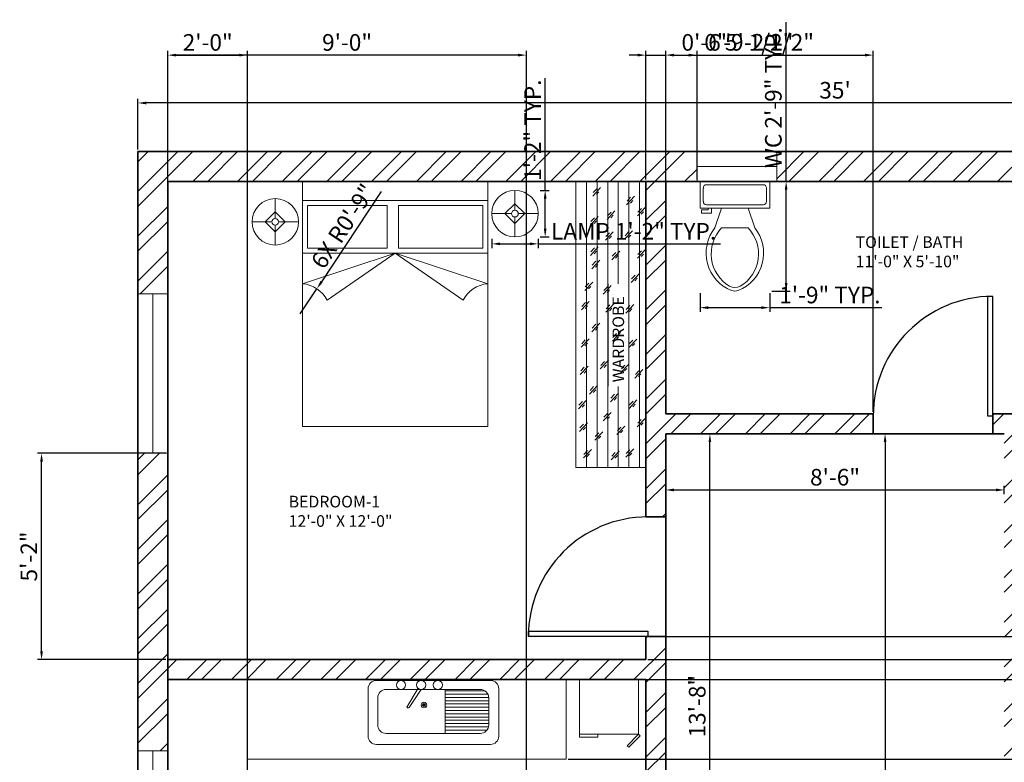
# Model space of a CAD drawing. Units: inches. Extents: x 28986 to 29505, y -162 to 451.
# Tile 5 of 6: x 29016 to 29312, y 228 to 451. Entities that reach past the tile are written whole.
import ezdxf

# ---------------------------------------------------------------- set-up
doc = ezdxf.new("R2010")
doc.units = ezdxf.units.IN
doc.layers.get('Defpoints').update_dxf_attribs({"color": 120})
for name, color, linetype, lineweight, true_color in [('A-ANNO-DIMS', 9, 'Continuous', 18, 0xafd9aa), ('A-FLOR-CASE', 32, 'Continuous', 18, 0xcd6928), ('A-FLOR-CASE-PATT', 32, 'Continuous', 13, 0xcd6928)]:
    doc.layers.add(name, color=color, linetype=linetype, lineweight=lineweight, true_color=true_color)
for name, color, linetype, lineweight in [('A-ANNO-TEXT', 6, 'Continuous', 18), ('A-AREA-IDEN', 6, 'Continuous', 18), ('A-EQPM', 8, 'Continuous', 18), ('A-FLOR-FIXT', 9, 'Continuous', 18), ('A-GLAZ', 4, 'Continuous', 18), ('A-WALL', 7, 'Continuous', 35), ('A-WALL-PATT', 1, 'Continuous', 13), ('DOOR', 2, 'Continuous', 25), ('FURNITURE', 241, 'Continuous', 18)]:
    doc.layers.add(name, color=color, linetype=linetype, lineweight=lineweight)
doc.styles.get("Standard").update_dxf_attribs({"font": 'arial.ttf'})
doc.dimstyles.new('ISO-25', dxfattribs={"dimtxt": 5, "dimasz": 2.5, "dimexe": 1.25, "dimexo": 0.625, "dimtad": 1, "dimdec": 0, "dimlunit": 3, "dimtxsty": 'Standard', "dimcen": 2.5, "dimadec": 0, "dimazin": 0, "dimtfac": 1, "dimtdec": 0, "dimtmove": 0, "dimatfit": 3, "dimfxl": 1, "dimarcsym": 0})

# ---------------------------------------------------------------- blocks, each defined once
blk = doc.blocks.new('*U5')
for p, q in [((0, 0), (0, -6)), ((-40, 0), (-40, -6))]:
    blk.add_line(p, q)
blk.add_lwpolyline([(0, 0), (0, 40), (-1.75, 40), (-1.75, 0)], close=True)
blk.add_arc((0, 0), 40, 90, 180)
blk = doc.blocks.new('*U6')
for p, q in [((0, 0), (0, -6)), ((40, 0), (40, -6))]:
    blk.add_line(p, q)
blk.add_lwpolyline([(0, 0), (0, 40), (1.75, 40), (1.75, 0)], close=True)
blk.add_arc((0, 0), 40, 0, 90)
blk = doc.blocks.new('modern bed')
for p, q in [((-55.85, 73.76), (-55.85, 0)), ((0, 0), (0, 73.76)), ((-55.85, 68.07), (0, 68.07)), ((-54.35, 66.57), (-54.35, 53.68)), ((-54.35, 66.57), (-30.33, 66.57)), ((-30.33, 66.57), (-30.33, 53.68)), ((-26.87, 66.57), (-1.5, 66.57)), ((-26.87, 66.57), (-26.87, 53.68)), ((-1.5, 53.68), (-1.5, 66.57)), ((-54.35, 53.68), (-30.33, 53.68)), ((-26.87, 53.68), (-1.5, 53.68)), ((-55.85, 52.18), (0, 52.18)), ((-27.93, 52.18), (-55.85, 42.95)), ((-27.93, 52.18), (-48.41, 38.03)), ((-27.93, 52.18), (0, 42.95)), ((-27.93, 52.18), (-7.44, 38.03)), ((-55.85, 0), (0, 0))]:
    blk.add_line(p, q)
blk.add_lwpolyline([(-55.85, 73.76), (0, 73.76)])
for centre, start, end in [((-56.5, 33.89), 27.0819, 85.9278), ((0.64, 33.89), 94.0722, 152.9181)]:
    blk.add_arc(centre, 9.08, start, end)
blk = doc.blocks.new('sink')
for p, q in [((-11.38, 27.19), (-5.63, 30.57)), ((-11.01, 26.26), (-5.62, 29.92)), ((-11.03, 19), (2.23, 19)), ((-10.58, 19), (-10.58, 7)), ((-9.6, 19), (-9.6, 6.16)), ((-8.61, 19), (-8.61, 5.92)), ((-7.63, 19), (-7.63, 5.92)), ((-6.64, 19), (-6.64, 5.92)), ((-5.66, 19), (-5.66, 5.92)), ((-4.67, 19), (-4.67, 5.92)), ((-3.69, 19), (-3.69, 5.92)), ((-2.7, 19), (-2.7, 5.92)), ((-1.72, 19), (-1.72, 5.92)), ((-0.73, 19), (-0.73, 5.92)), ((0.25, 19), (0.25, 5.98)), ((1.23, 19), (1.23, 6.43))]:
    blk.add_line(p, q)
for points in [[(-11.21, 42.26), (3.04, 42.26, -0.414214), (5.54, 39.76), (5.54, 5.38, -0.414214), (3.04, 2.88), (-11.21, 2.88, -0.414214), (-13.71, 5.38), (-13.71, 39.76, -0.414214)], [(-8.53, 39.31), (-0.27, 39.31, -0.414214), (2.23, 36.81), (2.23, 8.42, -0.414214), (-0.27, 5.92), (-8.53, 5.92, -0.414214), (-11.03, 8.42), (-11.03, 36.81, -0.414214)]]:
    blk.add_lwpolyline(points, format="xyb", close=True)
for centre, radius in [((-12.38, 32.33), 1.37), ((-12.38, 26.26), 1.37), ((-6.32, 25.41), 0.854), ((-6.32, 25.41), 0.432), ((-6.32, 25.41), 0.203), ((-12.38, 21.24), 1.37)]:
    blk.add_circle(centre, radius)
blk.add_arc((-5.86, 30.24), 0.398, 306.1138, 55.3114)
blk = doc.blocks.new('Lamp - Table')
for p, q in [((0, 7), (0, 1)), ((0, 3), (-3, 0)), ((3, 0), (0, 3)), ((-1, 0), (-7, 0)), ((-3, 0), (0, -3)), ((0, -3), (3, 0)), ((1, 0), (7, 0)), ((0, -1), (0, -7))]:
    blk.add_line(p, q)
for radius in [7, 1]:
    blk.add_circle((0, 0), radius)
blk = doc.blocks.new('*D18')
at = {"layer": 'A-ANNO-DIMS', "color": 0, "lineweight": -2, "transparency": 16777216}
for p, q in [((29278.83, 326.7), (29274.99, 326.7)), ((29276.24, 324.2), (29276.24, -62.8)), ((29278.83, -65.3), (29274.99, -65.3))]:
    blk.add_line(p, q, dxfattribs=at)
at = {"layer": 'A-ANNO-DIMS', "color": 0, "transparency": 16777216}
for points in [[(29275.82, 324.2), (29276.65, 324.2), (29276.24, 326.7)], [(29275.82, -62.8), (29276.65, -62.8), (29276.24, -65.3)]]:
    blk.add_solid(points, dxfattribs=at)
at = {"layer": 'Defpoints', "color": 0, "transparency": 16777216}
for p in [(29279.46, 326.7), (29276.24, -65.3), (29279.46, -65.3)]:
    blk.add_point(p, dxfattribs=at)
at = {"layer": 'A-ANNO-DIMS', "color": 0, "transparency": 16777216, "insert": (29273.06, 130.7), "char_height": 5, "attachment_point": 5, "rotation": 90}
blk.add_mtext('32\'-8"', dxfattribs=at)
blk = doc.blocks.new('FRIDGE')
for points in [[(0, 16.47), (17.77, 16.47), (17.77, 0), (0, 0)], [(0, 0), (5.53, 0), (5.53, -0.88), (0, -0.88)], [(18.23, -0.47), (17.77, 0), (14.32, -3.43), (14.79, -3.9)]]:
    blk.add_lwpolyline(points, close=True)
blk = doc.blocks.new('*D22')
at = {"layer": 'A-ANNO-DIMS', "color": 0, "lineweight": -2, "transparency": 16777216}
for p, q in [((29210.78, 326.7), (29224.71, 326.7)), ((29223.46, 165.2), (29223.46, 324.2)), ((29210.78, 162.7), (29224.71, 162.7))]:
    blk.add_line(p, q, dxfattribs=at)
at = {"layer": 'A-ANNO-DIMS', "color": 0, "transparency": 16777216}
for points in [[(29223.04, 324.2), (29223.87, 324.2), (29223.46, 326.7)], [(29223.04, 165.2), (29223.87, 165.2), (29223.46, 162.7)]]:
    blk.add_solid(points, dxfattribs=at)
at = {"layer": 'Defpoints', "color": 0, "transparency": 16777216}
for p in [(29210.16, 326.7), (29223.46, 326.7), (29210.16, 162.7)]:
    blk.add_point(p, dxfattribs=at)
at = {"layer": 'A-ANNO-DIMS', "color": 0, "transparency": 16777216, "insert": (29220.28, 244.7), "char_height": 5, "attachment_point": 5, "rotation": 90}
blk.add_mtext('13\'-8"', dxfattribs=at)
blk = doc.blocks.new('Toilet - top')
for p, q in [((9.5, -6), (9.5, -2)), ((-10, -8.5), (-8, -8.5)), ((-10, -9.5), (-10, -8.5)), ((-8, -8.5), (-8, -8)), ((-7, -8), (-7, -9.5)), ((-4, -8), (-6, -14)), ((4, -8), (6, -14)), ((-7, -9.5), (-10, -9.5)), ((4, -14), (-4, -14))]:
    blk.add_line(p, q)
blk.add_lwpolyline([(10.5, -8), (10.5, 0), (-10.5, 0), (-10.5, -8)], close=True)
for points in [[(-9.5, -2), (-9.5, -6)], [(8.5, -1), (-8.5, -1)], [(-8.5, -7), (8.5, -7)]]:
    blk.add_lwpolyline(points)
for centre, radius, start, end in [((-8.62, -1.88), 0.884, 81.8699, 188.1301), ((8.62, -1.88), 0.884, 351.8699, 98.1301), ((-8.62, -6.12), 0.884, 171.8699, 278.1301), ((8.62, -6.12), 0.884, 261.8699, 8.1301), ((3.52, -21.58), 12.17, 141.4691, 247.9714), ((4.2, -21.82), 11.33, 136.3677, 238.9468), ((-3.52, -21.58), 12.17, 292.0284, 38.5307), ((-4.2, -21.82), 11.33, 301.053, 43.6321), ((0, -27.88), 4, 245.7318, 294.2682), ((0, -29), 4, 254.8605, 285.1395)]:
    blk.add_arc(centre, radius, start, end)
blk = doc.blocks.new('*D24')
at = {"layer": 'A-ANNO-DIMS', "color": 0, "lineweight": -2, "transparency": 16777216}
for p, q in [((29210.16, 308.53), (29210.16, 311.06)), ((29212.66, 309.81), (29309.66, 309.81)), ((29312.16, 308.53), (29312.16, 311.06))]:
    blk.add_line(p, q, dxfattribs=at)
at = {"layer": 'A-ANNO-DIMS', "color": 0, "transparency": 16777216}
for points in [[(29212.66, 310.23), (29212.66, 309.39), (29210.16, 309.81)], [(29309.66, 310.23), (29309.66, 309.39), (29312.16, 309.81)]]:
    blk.add_solid(points, dxfattribs=at)
at = {"layer": 'Defpoints', "color": 0, "transparency": 16777216}
for p in [(29312.16, 309.81), (29210.16, 307.91), (29312.16, 307.91)]:
    blk.add_point(p, dxfattribs=at)
at = {"layer": 'A-ANNO-DIMS', "color": 0, "transparency": 16777216, "insert": (29261.16, 312.99), "char_height": 5, "attachment_point": 5}
blk.add_mtext('8\'-6"', dxfattribs=at)
blk = doc.blocks.new('*D25')
at = {"layer": 'A-ANNO-DIMS', "color": 0, "lineweight": -2, "transparency": 16777216}
for p, q in [((29051.16, 412.32), (29051.16, 427.59)), ((29471.16, 412.32), (29471.16, 427.59)), ((29468.66, 426.34), (29053.66, 426.34))]:
    blk.add_line(p, q, dxfattribs=at)
at = {"layer": 'A-ANNO-DIMS', "color": 0, "transparency": 16777216}
for points in [[(29053.66, 426.75), (29053.66, 425.92), (29051.16, 426.34)], [(29468.66, 426.75), (29468.66, 425.92), (29471.16, 426.34)]]:
    blk.add_solid(points, dxfattribs=at)
at = {"layer": 'Defpoints', "color": 0, "transparency": 16777216}
for p in [(29051.16, 426.34), (29051.16, 411.7), (29471.16, 411.7)]:
    blk.add_point(p, dxfattribs=at)
at = {"layer": 'A-ANNO-DIMS', "color": 0, "transparency": 16777216, "insert": (29261.16, 429.52), "char_height": 5, "attachment_point": 5}
blk.add_mtext("35'", dxfattribs=at)
blk = doc.blocks.new('WIN-48IN')
for p, q in [((9, 48), (0, 48)), ((4.5, 0), (4.5, 48)), ((9, 0), (0, 0))]:
    blk.add_line(p, q)
blk = doc.blocks.new('WIN-24IN')
for p, q in [((0, 0), (0, 9)), ((24, 0), (24, 9)), ((0, 4.5), (24, 4.5))]:
    blk.add_line(p, q)
blk = doc.blocks.new('WARDROBE-86IN')
for p, q in [((2.83, 18.79), (5.37, 16.41)), ((3.92, 18.65), (5.05, 17.57)), ((10.82, 19.98), (13.37, 17.6)), ((11.31, 18.86), (12.06, 18.15)), ((11.91, 19.85), (13.04, 18.77)), ((17.6, 20.32), (20.15, 17.94)), ((18.09, 19.2), (18.84, 18.49)), ((18.69, 20.18), (19.82, 19.11)), ((27.93, 19.75), (30.48, 17.37)), ((28.42, 18.62), (29.17, 17.91)), ((29.03, 19.61), (30.15, 18.53)), ((36.16, 19.46), (38.7, 17.08)), ((36.65, 18.33), (37.39, 17.62)), ((37.25, 19.32), (38.38, 18.24)), ((47.4, 19.42), (49.95, 17.04)), ((47.89, 18.3), (48.64, 17.59)), ((48.5, 19.29), (49.62, 18.21)), ((53.27, 18.39), (55.81, 16.01)), ((54.36, 18.25), (55.49, 17.17)), ((3.32, 17.66), (4.06, 16.95)), ((8.19, 15.38), (10.73, 13)), ((9.28, 15.24), (10.41, 14.16)), ((22.1, 16.94), (24.65, 14.56)), ((22.59, 15.82), (23.34, 15.1)), ((23.2, 16.8), (24.32, 15.72)), ((40.87, 16.28), (43.41, 13.9)), ((41.36, 15.15), (42.1, 14.44)), ((41.96, 16.14), (43.09, 15.06)), ((53.76, 17.27), (54.5, 16.55)), ((59.84, 16.27), (62.39, 13.89)), ((60.33, 15.14), (61.08, 14.43)), ((60.94, 16.13), (62.06, 15.05)), ((63.85, 16.72), (66.39, 14.34)), ((64.34, 15.6), (65.08, 14.88)), ((64.94, 16.58), (66.07, 15.5)), ((72.96, 16.7), (75.51, 14.32)), ((73.45, 15.57), (74.2, 14.86)), ((74.06, 16.56), (75.18, 15.48)), ((81.71, 16.01), (84.25, 13.63)), ((82.2, 14.88), (82.95, 14.17)), ((82.8, 15.87), (83.93, 14.79)), ((8.68, 14.26), (9.42, 13.54)), ((14, 12.81), (16.55, 10.43)), ((15.1, 12.67), (16.22, 11.59)), ((29.63, 13.72), (32.17, 11.34)), ((30.11, 12.59), (30.86, 11.88)), ((30.72, 13.58), (31.85, 12.5)), ((46.7, 12.07), (49.24, 9.69)), ((47.79, 11.93), (48.92, 10.85)), ((52.19, 12.81), (54.74, 10.43)), ((53.29, 12.67), (54.41, 11.59)), ((68.4, 12.2), (70.94, 9.82)), ((69.49, 12.07), (70.62, 10.99)), ((2.31, 10.42), (4.85, 8.04)), ((2.79, 9.29), (3.54, 8.58)), ((3.4, 10.28), (4.53, 9.2)), ((14.49, 11.68), (15.24, 10.97)), ((19.79, 10.66), (22.34, 8.28)), ((20.28, 9.54), (21.03, 8.82)), ((20.88, 10.52), (22.01, 9.44)), ((38.06, 10.04), (40.6, 7.66)), ((38.55, 8.92), (39.29, 8.2)), ((39.15, 9.9), (40.28, 8.82)), ((47.19, 10.94), (47.93, 10.23)), ((52.68, 11.68), (53.43, 10.97)), ((62.53, 10.24), (65.07, 7.86)), ((63.02, 9.12), (63.76, 8.4)), ((63.62, 10.1), (64.75, 9.02)), ((68.89, 11.08), (69.63, 10.37)), ((74.68, 11.68), (77.23, 9.3)), ((75.17, 10.55), (75.92, 9.84)), ((75.77, 11.54), (76.9, 10.46)), ((3.05, 6.03), (5.59, 3.65)), ((9.91, 8.72), (12.45, 6.34)), ((10.4, 7.6), (11.15, 6.88)), ((11, 8.58), (12.13, 7.5)), ((28.55, 7.52), (31.1, 5.14)), ((29.04, 6.4), (29.79, 5.68)), ((29.65, 7.38), (30.77, 6.3)), ((46.49, 6.03), (49.03, 3.65)), ((68.68, 6.41), (71.23, 4.03)), ((69.78, 6.27), (70.9, 5.19)), ((3.54, 4.91), (4.28, 4.2)), ((4.14, 5.89), (5.27, 4.82)), ((17.77, 5.05), (20.31, 2.67)), ((18.25, 3.92), (19, 3.21)), ((18.86, 4.91), (19.99, 3.83)), ((26.9, 3.3), (29.44, 0.92)), ((27.99, 3.16), (29.12, 2.08)), ((36.07, 5.13), (38.62, 2.75)), ((36.56, 4), (37.31, 3.29)), ((37.17, 4.99), (38.29, 3.91)), ((46.97, 4.9), (47.72, 4.19)), ((47.58, 5.89), (48.71, 4.81)), ((55.71, 4.42), (58.25, 2.04)), ((56.2, 3.29), (56.94, 2.58)), ((56.8, 4.28), (57.93, 3.2)), ((69.17, 5.28), (69.92, 4.57)), ((79.11, 5.8), (81.65, 3.42)), ((79.6, 4.67), (80.34, 3.96)), ((80.2, 5.66), (81.33, 4.58)), ((12.18, 2.6), (14.73, 0.22)), ((12.67, 1.47), (13.42, 0.76)), ((13.28, 2.46), (14.4, 1.38)), ((27.39, 2.18), (28.13, 1.46)), ((62.98, 2.55), (65.52, 0.17)), ((63.47, 1.43), (64.21, 0.72)), ((64.07, 2.42), (65.2, 1.34)), ((75.74, 2.55), (78.28, 0.17)), ((76.23, 1.43), (76.97, 0.72)), ((76.83, 2.42), (77.96, 1.34))]:
    blk.add_line(p, q)
blk.add_lwpolyline([(86.1, 21.04), (0, 21.04), (0, 0), (86.1, 0)], close=True)
blk = doc.blocks.new('*D35')
at = {"layer": 'A-ANNO-DIMS', "color": 0, "lineweight": -2, "transparency": 16777216}
for p, q in [((29157.73, 385.39), (29157.73, 382.66)), ((29160.23, 383.91), (29169.23, 383.91)), ((29171.73, 385.39), (29171.73, 382.66)), ((29171.73, 383.91), (29226.7, 383.91))]:
    blk.add_line(p, q, dxfattribs=at)
at = {"layer": 'A-ANNO-DIMS', "color": 0, "transparency": 16777216}
for points in [[(29160.23, 384.33), (29160.23, 383.5), (29157.73, 383.91)], [(29169.23, 384.33), (29169.23, 383.5), (29171.73, 383.91)]]:
    blk.add_solid(points, dxfattribs=at)
at = {"layer": 'Defpoints', "color": 0, "transparency": 16777216}
for p in [(29157.73, 386.01), (29171.73, 386.01), (29171.73, 383.91)]:
    blk.add_point(p, dxfattribs=at)
at = {"layer": 'A-ANNO-DIMS', "color": 0, "transparency": 16777216, "insert": (29200.47, 387.05), "char_height": 5, "attachment_point": 5}
blk.add_mtext('LAMP 1\'-2" TYP.', dxfattribs=at)
blk = doc.blocks.new('*D36')
at = {"layer": 'A-ANNO-DIMS', "color": 0, "lineweight": -2, "transparency": 16777216}
for p, q in [((29173.83, 400.01), (29173.83, 433.77)), ((29172.36, 400.01), (29175.08, 400.01)), ((29173.83, 388.51), (29173.83, 397.51)), ((29172.36, 386.01), (29175.08, 386.01))]:
    blk.add_line(p, q, dxfattribs=at)
at = {"layer": 'A-ANNO-DIMS', "color": 0, "transparency": 16777216}
for points in [[(29173.42, 397.51), (29174.25, 397.51), (29173.83, 400.01)], [(29173.42, 388.51), (29174.25, 388.51), (29173.83, 386.01)]]:
    blk.add_solid(points, dxfattribs=at)
at = {"layer": 'Defpoints', "color": 0, "transparency": 16777216}
for p in [(29171.73, 400.01), (29173.83, 400.01), (29171.73, 386.01)]:
    blk.add_point(p, dxfattribs=at)
at = {"layer": 'A-ANNO-DIMS', "color": 0, "transparency": 16777216, "insert": (29170.7, 418.14), "char_height": 5, "attachment_point": 5, "rotation": 90}
blk.add_mtext('1\'-2" TYP.', dxfattribs=at)
blk = doc.blocks.new('*D53')
at = {"layer": 'A-ANNO-DIMS', "color": 0, "lineweight": -2, "transparency": 16777216}
for p, q in [((29246.43, 402.7), (29246.43, 450.71)), ((29242.1, 402.7), (29247.68, 402.7)), ((29246.43, 372.15), (29246.43, 400.2)), ((29242.1, 369.65), (29247.68, 369.65))]:
    blk.add_line(p, q, dxfattribs=at)
at = {"layer": 'A-ANNO-DIMS', "color": 0, "transparency": 16777216}
for points in [[(29246.02, 400.2), (29246.85, 400.2), (29246.43, 402.7)], [(29246.02, 372.15), (29246.85, 372.15), (29246.43, 369.65)]]:
    blk.add_solid(points, dxfattribs=at)
at = {"layer": 'Defpoints', "color": 0, "transparency": 16777216}
for p in [(29241.48, 402.7), (29246.43, 402.7), (29241.48, 369.65)]:
    blk.add_point(p, dxfattribs=at)
at = {"layer": 'A-ANNO-DIMS', "color": 0, "transparency": 16777216, "insert": (29243.22, 427.95), "char_height": 5, "attachment_point": 5, "rotation": 90}
blk.add_mtext('WC 2\'-9" TYP.', dxfattribs=at)
blk = doc.blocks.new('*D54')
at = {"layer": 'A-ANNO-DIMS', "color": 0, "lineweight": -2, "transparency": 16777216}
for p, q in [((29220.48, 369.03), (29220.48, 363.45)), ((29241.48, 369.03), (29241.48, 363.45)), ((29222.98, 364.7), (29238.98, 364.7)), ((29241.48, 364.7), (29275.23, 364.7))]:
    blk.add_line(p, q, dxfattribs=at)
at = {"layer": 'A-ANNO-DIMS', "color": 0, "transparency": 16777216}
for points in [[(29222.98, 365.11), (29222.98, 364.28), (29220.48, 364.7)], [(29238.98, 365.11), (29238.98, 364.28), (29241.48, 364.7)]]:
    blk.add_solid(points, dxfattribs=at)
at = {"layer": 'Defpoints', "color": 0, "transparency": 16777216}
for p in [(29220.48, 369.65), (29241.48, 369.65), (29241.48, 364.7)]:
    blk.add_point(p, dxfattribs=at)
at = {"layer": 'A-ANNO-DIMS', "color": 0, "transparency": 16777216, "insert": (29259.6, 367.87), "char_height": 5, "attachment_point": 5}
blk.add_mtext('1\'-9" TYP.', dxfattribs=at)
blk = doc.blocks.new('*D64')
at = {"layer": 'A-ANNO-DIMS', "color": 0, "lineweight": -2, "transparency": 16777216}
for p, q in [((29060.16, 26.32), (29060.16, 442)), ((29168.16, 26.32), (29168.16, 442)), ((29165.66, 440.75), (29062.66, 440.75))]:
    blk.add_line(p, q, dxfattribs=at)
at = {"layer": 'A-ANNO-DIMS', "color": 0, "transparency": 16777216}
for points in [[(29062.66, 441.17), (29062.66, 440.33), (29060.16, 440.75)], [(29165.66, 441.17), (29165.66, 440.33), (29168.16, 440.75)]]:
    blk.add_solid(points, dxfattribs=at)
at = {"layer": 'Defpoints', "color": 0, "transparency": 16777216}
for p in [(29060.16, 440.75), (29060.16, 25.7), (29168.16, 25.7)]:
    blk.add_point(p, dxfattribs=at)
at = {"layer": 'A-ANNO-DIMS', "color": 0, "transparency": 16777216, "insert": (29114.16, 443.93), "char_height": 5, "attachment_point": 5}
blk.add_mtext('9\'-0"', dxfattribs=at)
blk = doc.blocks.new('*D66')
at = {"layer": 'A-ANNO-DIMS', "color": 0, "lineweight": -2, "transparency": 16777216}
for p, q in [((29210.16, 403.32), (29210.16, 442)), ((29219.6, 403.32), (29219.6, 442)), ((29212.66, 440.75), (29217.1, 440.75)), ((29219.6, 440.75), (29248.3, 440.75))]:
    blk.add_line(p, q, dxfattribs=at)
at = {"layer": 'A-ANNO-DIMS', "color": 0, "transparency": 16777216}
for points in [[(29212.66, 441.17), (29212.66, 440.33), (29210.16, 440.75)], [(29217.1, 441.17), (29217.1, 440.33), (29219.6, 440.75)]]:
    blk.add_solid(points, dxfattribs=at)
at = {"layer": 'Defpoints', "color": 0, "transparency": 16777216}
for p in [(29219.6, 440.75), (29210.16, 402.7), (29219.6, 402.7)]:
    blk.add_point(p, dxfattribs=at)
at = {"layer": 'A-ANNO-DIMS', "color": 0, "transparency": 16777216, "insert": (29235.2, 443.96), "char_height": 5, "attachment_point": 5}
blk.add_mtext('0\'-9 1/2"', dxfattribs=at)
blk = doc.blocks.new('*D70')
at = {"layer": 'A-ANNO-DIMS', "color": 0, "lineweight": -2, "transparency": 16777216}
for p, q in [((29059.53, 320.84), (29020.86, 320.84)), ((29022.11, 261.2), (29022.11, 318.34)), ((29059.53, 258.7), (29020.86, 258.7))]:
    blk.add_line(p, q, dxfattribs=at)
at = {"layer": 'A-ANNO-DIMS', "color": 0, "transparency": 16777216}
for points in [[(29021.69, 318.34), (29022.52, 318.34), (29022.11, 320.84)], [(29021.69, 261.2), (29022.52, 261.2), (29022.11, 258.7)]]:
    blk.add_solid(points, dxfattribs=at)
at = {"layer": 'Defpoints', "color": 0, "transparency": 16777216}
for p in [(29022.11, 320.84), (29060.16, 320.84), (29060.16, 258.7)]:
    blk.add_point(p, dxfattribs=at)
at = {"layer": 'A-ANNO-DIMS', "color": 0, "transparency": 16777216, "insert": (29018.93, 289.77), "char_height": 5, "attachment_point": 5, "rotation": 90}
blk.add_mtext('5\'-2"', dxfattribs=at)
blk = doc.blocks.new('*D78')
at = {"layer": 'A-ANNO-DIMS', "color": 0, "lineweight": -2, "transparency": 16777216}
for p, q in [((29204.16, 403.32), (29204.16, 442)), ((29210.16, 403.32), (29210.16, 442)), ((29201.66, 440.75), (29199.16, 440.75)), ((29204.16, 440.75), (29210.16, 440.75)), ((29212.66, 440.75), (29229.7, 440.75))]:
    blk.add_line(p, q, dxfattribs=at)
at = {"layer": 'A-ANNO-DIMS', "color": 0, "transparency": 16777216}
for points in [[(29201.66, 441.17), (29201.66, 440.33), (29204.16, 440.75)], [(29212.66, 441.17), (29212.66, 440.33), (29210.16, 440.75)]]:
    blk.add_solid(points, dxfattribs=at)
at = {"layer": 'Defpoints', "color": 0, "transparency": 16777216}
for p in [(29210.16, 440.75), (29204.16, 402.7), (29210.16, 402.7)]:
    blk.add_point(p, dxfattribs=at)
at = {"layer": 'A-ANNO-DIMS', "color": 0, "transparency": 16777216, "insert": (29222.43, 443.93), "char_height": 5, "attachment_point": 5}
blk.add_mtext('0\'-6"', dxfattribs=at)
blk = doc.blocks.new('*D81')
at = {"layer": 'A-ANNO-DIMS', "color": 0, "lineweight": -2, "transparency": 16777216}
for p, q in [((29210.16, 333.32), (29210.16, 442)), ((29272.66, 333.32), (29272.66, 442)), ((29212.66, 440.75), (29270.16, 440.75))]:
    blk.add_line(p, q, dxfattribs=at)
at = {"layer": 'A-ANNO-DIMS', "color": 0, "transparency": 16777216}
for points in [[(29212.66, 441.17), (29212.66, 440.33), (29210.16, 440.75)], [(29270.16, 441.17), (29270.16, 440.33), (29272.66, 440.75)]]:
    blk.add_solid(points, dxfattribs=at)
at = {"layer": 'Defpoints', "color": 0, "transparency": 16777216}
for p in [(29272.66, 440.75), (29210.16, 332.7), (29272.66, 332.7)]:
    blk.add_point(p, dxfattribs=at)
at = {"layer": 'A-ANNO-DIMS', "color": 0, "transparency": 16777216, "insert": (29241.41, 443.96), "char_height": 5, "attachment_point": 5}
blk.add_mtext('5\'-2 1/2"', dxfattribs=at)
blk = doc.blocks.new('*D85')
at = {"layer": 'A-ANNO-DIMS', "color": 0, "lineweight": -2, "transparency": 16777216}
for p, q in [((29500.21, 265.69), (29500.21, 282.73)), ((29204.78, 265.69), (29501.46, 265.69)), ((29500.21, 261.2), (29500.21, 263.19)), ((29204.78, 258.7), (29501.46, 258.7))]:
    blk.add_line(p, q, dxfattribs=at)
at = {"layer": 'A-ANNO-DIMS', "color": 0, "transparency": 16777216}
for points in [[(29499.79, 263.19), (29500.62, 263.19), (29500.21, 265.69)], [(29499.79, 261.2), (29500.62, 261.2), (29500.21, 258.7)]]:
    blk.add_solid(points, dxfattribs=at)
at = {"layer": 'Defpoints', "color": 0, "transparency": 16777216}
for p in [(29204.16, 265.69), (29500.21, 265.69), (29204.16, 258.7)]:
    blk.add_point(p, dxfattribs=at)
at = {"layer": 'A-ANNO-DIMS', "color": 0, "transparency": 16777216, "insert": (29497.03, 275.46), "char_height": 5, "attachment_point": 5, "rotation": 90}
blk.add_mtext('0\'-7"', dxfattribs=at)
blk = doc.blocks.new('*D88')
at = {"layer": 'A-ANNO-DIMS', "color": 0, "lineweight": -2, "transparency": 16777216}
for p, q in [((29060.16, -16.69), (29060.16, 442)), ((29084.16, -16.69), (29084.16, 442)), ((29062.66, 440.75), (29081.66, 440.75))]:
    blk.add_line(p, q, dxfattribs=at)
at = {"layer": 'A-ANNO-DIMS', "color": 0, "transparency": 16777216}
for points in [[(29062.66, 441.17), (29062.66, 440.33), (29060.16, 440.75)], [(29081.66, 441.17), (29081.66, 440.33), (29084.16, 440.75)]]:
    blk.add_solid(points, dxfattribs=at)
at = {"layer": 'Defpoints', "color": 0, "transparency": 16777216}
for p in [(29084.16, 440.75), (29060.16, -17.32), (29084.16, -17.32)]:
    blk.add_point(p, dxfattribs=at)
at = {"layer": 'A-ANNO-DIMS', "color": 0, "transparency": 16777216, "insert": (29072.16, 443.93), "char_height": 5, "attachment_point": 5}
blk.add_mtext('2\'-0"', dxfattribs=at)
blk = doc.blocks.new('*D97')
at = {"layer": 'A-ANNO-DIMS', "color": 0, "lineweight": -2, "transparency": 16777216}
for p, q in [((29180.78, 252.7), (29501.46, 252.7)), ((29500.21, 231.2), (29500.21, 250.2)), ((29180.78, 228.7), (29501.46, 228.7))]:
    blk.add_line(p, q, dxfattribs=at)
at = {"layer": 'A-ANNO-DIMS', "color": 0, "transparency": 16777216}
for points in [[(29499.79, 250.2), (29500.62, 250.2), (29500.21, 252.7)], [(29499.79, 231.2), (29500.62, 231.2), (29500.21, 228.7)]]:
    blk.add_solid(points, dxfattribs=at)
at = {"layer": 'Defpoints', "color": 0, "transparency": 16777216}
for p in [(29180.16, 252.7), (29500.21, 252.7), (29180.16, 228.7)]:
    blk.add_point(p, dxfattribs=at)
at = {"layer": 'A-ANNO-DIMS', "color": 0, "transparency": 16777216, "insert": (29497.03, 240.7), "char_height": 5, "attachment_point": 5, "rotation": 90}
blk.add_mtext('2\'-0"', dxfattribs=at)
blk = doc.blocks.new('*D103')
at = {"layer": 'A-ANNO-DIMS', "color": 0, "lineweight": -2, "transparency": 16777216}
for p, q in [((29124.44, 399.67), (29106.45, 372.49)), ((29100.06, 362.83), (29105.07, 370.4))]:
    blk.add_line(p, q, dxfattribs=at)
at = {"layer": 'A-ANNO-DIMS', "color": 0, "transparency": 16777216}
blk.add_solid([(29106.1, 372.72), (29106.8, 372.26), (29105.07, 370.4)], dxfattribs=at)
at = {"layer": 'Defpoints', "color": 0, "transparency": 16777216}
for p in [(29105.07, 370.4), (29100.06, 362.83)]:
    blk.add_point(p, dxfattribs=at)
at = {"layer": 'A-ANNO-DIMS', "color": 0, "transparency": 16777216, "insert": (29113.49, 388.88), "char_height": 5, "attachment_point": 5, "rotation": 56.5039}
blk.add_mtext('6X R0\'-9"', dxfattribs=at)

msp = doc.modelspace()

# ---------------------------------------------------------------- hatches: boundary and pattern name
at = {"layer": 'A-WALL-PATT'}
h = msp.add_hatch(dxfattribs=at)
h.set_pattern_fill('ANSI32', color=256)
h.paths.add_polyline_path([(29174.16, 34.7), (29163.04, 34.7), (29163.04, 29.3), (29163.04, 25.7), (29168.16, 25.7), (29168.16, -119.3), (29174.16, -119.3), (29174.16, -71.3), (29199.96, -71.3), (29199.96, -65.3), (29174.16, -65.3)])
h.paths.add_polyline_path([(29244.8, -65.3), (29235.96, -65.3), (29235.96, -71.3), (29244.8, -71.3)])
h.paths.add_polyline_path([(29318.16, 39.7), (29462.16, 39.7), (29462.16, 44.7), (29318.16, 44.7), (29318.16, 131.49), (29312.16, 131.49), (29312.16, -65.3), (29292.8, -65.3), (29292.8, -71.3), (29312.16, -71.3), (29312.16, -119.3), (29318.16, -119.3)])
h.paths.add_polyline_path([(29219.6, 411.7), (29051.16, 411.7), (29051.16, 368.84), (29060.16, 368.84), (29060.16, 402.7), (29204.16, 402.7), (29219.6, 402.7)])
h.paths.add_polyline_path([(29060.16, 320.84), (29051.16, 320.84), (29051.16, 231.24), (29060.16, 231.24), (29060.16, 252.7)])
h.paths.add_polyline_path([(29210.16, 265.69), (29204.76, 265.69), (29204.16, 265.69), (29204.16, 258.7), (29060.16, 258.7), (29060.16, 252.7), (29204.16, 252.7), (29204.16, 228.7), (29204.16, 168.7), (29199.96, 168.7), (29199.96, 167.47), (29199.96, 162.7), (29210.16, 162.7)])
h.paths.add_polyline_path([(29060.16, 183.24), (29051.16, 183.24), (29051.16, 162.7), (29060.16, 162.7), (29168.16, 162.7), (29168.16, 167.47), (29168.16, 168.7), (29060.16, 168.7)])
h.paths.add_polyline_path([(29060.16, 126.7), (29051.16, 126.7), (29051.16, 70.7), (29060.16, 70.7)])
h.paths.add_polyline_path([(29060.16, 25.7), (29127.04, 25.7), (29127.04, 34.7), (29060.16, 34.7), (29051.16, 34.7), (29051.16, -22.45), (29060.16, -22.45)])
h.paths.add_polyline_path([(29060.16, -70.45), (29051.16, -70.45), (29051.16, -128.3), (29084.16, -128.3), (29084.16, -119.3), (29060.16, -119.3)])
h.paths.add_polyline_path([(29174.16, -119.3), (29168.16, -119.3), (29132.16, -119.3), (29132.16, -128.3), (29174.16, -128.3)])
h.paths.add_polyline_path([(29471.16, 79.78), (29462.16, 79.78), (29462.16, -119.3), (29462.16, -128.3), (29471.16, -128.3)])
h.paths.add_polyline_path([(29462.16, 182.7), (29318.16, 182.7), (29318.16, 191.79), (29317.56, 191.79), (29312.16, 191.79), (29312.16, 167.49), (29317.56, 167.49), (29318.16, 167.49), (29318.16, 176.7), (29462.16, 176.7)])
h.paths.add_polyline_path([(29471.16, 221.37), (29462.16, 221.37), (29462.16, 135.64), (29471.16, 135.64)])
h.paths.add_polyline_path([(29471.16, 360.33), (29462.16, 360.33), (29462.16, 277.22), (29471.16, 277.22)])
h.paths.add_polyline_path([(29471.16, 411.7), (29243.6, 411.7), (29243.6, 402.7), (29462.16, 402.7), (29462.16, 384.33), (29471.16, 384.33)])
h.paths.add_polyline_path([(29348.16, 402.7), (29342.16, 402.7), (29342.16, 332.7), (29308.66, 332.7), (29308.66, 326.7), (29312.16, 326.7), (29312.16, 227.79), (29318.16, 227.79), (29318.16, 326.7), (29355.99, 326.7), (29355.99, 332.7), (29348.16, 332.7)])
h.paths.add_polyline_path([(29210.16, 326.7), (29272.66, 326.7), (29272.66, 332.1), (29272.66, 332.7), (29210.16, 332.7), (29210.16, 402.7), (29204.16, 402.7), (29204.16, 316.6), (29204.16, 301.69), (29210.16, 301.69)])

# ---------------------------------------------------------------- linework, layer by layer
at = {"layer": 'A-FLOR-CASE'}
for points in [[(29180.16, 252.7), (29180.16, 228.7)], [(29180.16, 252.7), (29204.16, 252.7)], [(29204.16, 252.7), (29204.16, 228.7)], [(29084.16, 168.7), (29084.16, 228.7), (29180.16, 228.7)]]:
    msp.add_lwpolyline(points, dxfattribs=at)
at = {"layer": 'A-WALL'}
for p, q in [((29471.16, 411.7), (29051.16, 411.7)), ((29051.16, 411.7), (29051.16, -128.3)), ((29462.16, 402.7), (29060.16, 402.7)), ((29060.16, 402.7), (29060.16, 168.7)), ((29204.16, 402.7), (29204.16, 301.69)), ((29210.16, 402.7), (29210.16, 332.7)), ((29272.66, 332.7), (29210.16, 332.7)), ((29272.66, 326.7), (29272.66, 332.7)), ((29342.16, 332.7), (29308.66, 332.7)), ((29308.66, 326.7), (29308.66, 332.7)), ((29210.16, 326.7), (29210.16, 162.7)), ((29312.16, 326.7), (29210.16, 326.7)), ((29204.16, 301.69), (29210.16, 301.69)), ((29204.16, 265.69), (29210.16, 265.69)), ((29204.16, 265.69), (29204.16, 258.7)), ((29204.16, 252.7), (29204.16, 168.7))]:
    msp.add_line(p, q, dxfattribs=at)
for points in [[(29204.16, 402.7), (29060.16, 402.7)], [(29204.16, 258.7), (29060.16, 258.7)], [(29204.16, 258.7), (29060.16, 258.7)], [(29204.16, 258.7), (29060.16, 258.7)], [(29204.16, 252.7), (29060.16, 252.7)], [(29060.16, 168.7), (29060.16, 252.7)]]:
    msp.add_lwpolyline(points, dxfattribs=at)

# ---------------------------------------------------------------- block references
at = {"layer": 'A-EQPM'}
msp.add_blockref('FRIDGE', (29184.21, 236.23), dxfattribs=at)
at = {"layer": 'A-FLOR-FIXT'}
msp.add_blockref('Toilet - top', (29230.98, 402.7), dxfattribs=at)
at = {"layer": 'A-FLOR-FIXT', "xscale": -1, "rotation": 90}
msp.add_blockref('sink', (29162.73, 238.72), dxfattribs=at)
at = {"layer": 'A-GLAZ'}
for name, p in [('WIN-24IN', (29219.6, 402.7)), ('WIN-48IN', (29051.16, 320.84)), ('WIN-48IN', (29051.16, 183.24))]:
    msp.add_blockref(name, p, dxfattribs=at)
at = {"layer": 'DOOR', "xscale": 0.8999999999999752, "yscale": 0.8999999999999752, "zscale": 0.8999999999999752}
msp.add_blockref('*U5', (29308.66, 332.1), dxfattribs=at)
at = {"layer": 'DOOR', "xscale": 0.8999999999999752, "yscale": 0.8999999999999752, "zscale": 0.8999999999999752, "rotation": 90}
msp.add_blockref('*U6', (29204.76, 265.69), dxfattribs=at)
at = {"layer": 'FURNITURE'}
for name, p in [('modern bed', (29156.56, 328.94)), ('Lamp - Table', (29092.52, 390.54)), ('Lamp - Table', (29164.73, 393.01))]:
    msp.add_blockref(name, p, dxfattribs=at)

# ---------------------------------------------------------------- texts
at = {"layer": 'A-AREA-IDEN', "char_height": 3.5, "attachment_point": 1}
for s, insert in [('TOILET / BATH\\P11\'-0" X 5\'-10"', (29267.37, 386.19)), ('BEDROOM-1\\P12\'-0" X 12\'-0"', (29096.56, 308.04))]:
    msp.add_mtext_dynamic_manual_height_columns(s, width=65.867, gutter_width=12.5, heights=[0], dxfattribs=dict(at, insert=insert))

# ---------------------------------------------------------------- dimensions: what is measured, and where the dimension line sits
at = {"layer": 'A-ANNO-DIMS'}
for base, p1, p2, override, picture, middle in [((29219.6, 440.75), (29210.16, 402.7), (29219.6, 402.7), {"dimdec": 1, "dimlfac": 1, "dimrnd": 0, "dimzin": 1, "dimdsep": 46, "dimlunit": 4, "dimfrac": 2}, '*D66', (29235.2, 443.96)), ((29272.66, 440.75), (29210.16, 332.7), (29272.66, 332.7), {"dimdec": 1, "dimlfac": 1, "dimrnd": 0, "dimzin": 1, "dimdsep": 46, "dimlunit": 4, "dimfrac": 2}, '*D81', (29241.41, 443.96)), ((29060.16, 440.75), (29168.16, 25.7), (29060.16, 25.7), {"dimdec": 1, "dimlfac": 1, "dimrnd": 0, "dimzin": 1, "dimdsep": 46, "dimlunit": 4, "dimfrac": 2}, '*D64', (29114.16, 443.93)), ((29084.16, 440.75), (29060.16, -17.32), (29084.16, -17.32), {"dimdec": 1, "dimlfac": 1, "dimrnd": 0, "dimzin": 1, "dimdsep": 46, "dimlunit": 4, "dimfrac": 2}, '*D88', (29072.16, 443.93)), ((29210.16, 440.75), (29204.16, 402.7), (29210.16, 402.7), {"dimdec": 1, "dimlfac": 1, "dimrnd": 0, "dimzin": 1, "dimdsep": 46, "dimlunit": 4, "dimfrac": 2}, '*D78', (29222.43, 443.93)), ((29051.16, 426.34), (29471.16, 411.7), (29051.16, 411.7), {"dimclrd": 0, "dimclre": 0, "dimclrt": 0}, '*D25', (29261.16, 429.52)), ((29312.16, 309.81), (29210.16, 307.91), (29312.16, 307.91), {"dimclrd": 0, "dimclre": 0, "dimclrt": 0}, '*D24', (29261.16, 312.99))]:
    dim = msp.add_linear_dim(base=base, p1=p1, p2=p2, dimstyle='ISO-25', override=override, dxfattribs=at)
    dim.commit()
    dim.dimension.update_dxf_attribs({"geometry": picture, "text_midpoint": middle})
for base, p1, p2, text, picture, middle in [((29246.433, 402.699), (29241.476, 369.6527), (29241.476, 402.699), 'WC <> TYP.', '*D53', (29243.2227, 427.9539)), ((29173.83, 400.01), (29171.73, 386.01), (29171.73, 400.01), '<> TYP.', '*D36', (29170.7, 418.14))]:
    dim = msp.add_linear_dim(base=base, p1=p1, p2=p2, angle=90, text=text, dimstyle='ISO-25', override={"dimdec": 1, "dimlfac": 1, "dimrnd": 0, "dimzin": 1, "dimdsep": 46, "dimlunit": 4, "dimfrac": 2}, dxfattribs=at)
    dim.commit()
    dim.dimension.update_dxf_attribs({"geometry": picture, "text_midpoint": middle})
dim = msp.add_radius_dim(center=(29100.06, 362.83), mpoint=(29105.07, 370.4), text='6X <>', dimstyle='ISO-25', override={"dimdec": 1, "dimlfac": 1, "dimrnd": 0, "dimzin": 1, "dimdsep": 46, "dimlunit": 4, "dimfrac": 2}, dxfattribs=at)
dim.commit()
dim.dimension.update_dxf_attribs({"geometry": '*D103', "text_midpoint": (29113.49, 388.88)})
for base, p1, p2, text, picture, middle in [((29171.73, 383.91), (29157.73, 386.01), (29171.73, 386.01), 'LAMP <> TYP.', '*D35', (29200.47, 387.05)), ((29241.48, 364.7), (29220.48, 369.65), (29241.48, 369.65), '<> TYP.', '*D54', (29259.6, 367.87))]:
    dim = msp.add_linear_dim(base=base, p1=p1, p2=p2, text=text, dimstyle='ISO-25', override={"dimdec": 1, "dimlfac": 1, "dimrnd": 0, "dimzin": 1, "dimdsep": 46, "dimlunit": 4, "dimfrac": 2}, dxfattribs=at)
    dim.commit()
    dim.dimension.update_dxf_attribs({"geometry": picture, "text_midpoint": middle})
for base, p1, p2, override, picture, middle in [((29223.46, 326.7), (29210.16, 162.7), (29210.16, 326.7), {"dimclrd": 0, "dimclre": 0, "dimclrt": 0}, '*D22', (29220.28, 244.7)), ((29276.24, -65.3), (29279.46, 326.7), (29279.46, -65.3), {"dimclrd": 0, "dimclre": 0, "dimclrt": 0}, '*D18', (29273.06, 130.7)), ((29022.11, 320.84), (29060.16, 258.7), (29060.16, 320.84), {"dimdec": 1, "dimlfac": 1, "dimrnd": 0, "dimzin": 1, "dimdsep": 46, "dimlunit": 4, "dimfrac": 2}, '*D70', (29018.93, 289.77)), ((29500.21, 265.69), (29204.16, 258.7), (29204.16, 265.69), {"dimdec": 1, "dimlfac": 1, "dimrnd": 0, "dimzin": 1, "dimdsep": 46, "dimlunit": 4, "dimfrac": 2}, '*D85', (29497.03, 275.46)), ((29500.21, 252.7), (29180.16, 228.7), (29180.16, 252.7), {"dimdec": 1, "dimlfac": 1, "dimrnd": 0, "dimzin": 1, "dimdsep": 46, "dimlunit": 4, "dimfrac": 2}, '*D97', (29497.03, 240.7))]:
    dim = msp.add_linear_dim(base=base, p1=p1, p2=p2, angle=90, dimstyle='ISO-25', override=override, dxfattribs=at)
    dim.commit()
    dim.dimension.update_dxf_attribs({"geometry": picture, "text_midpoint": middle})

# ---------------------------------------------------------------- next in the draw order: wipeouts: each hides what was drawn before it
msp.add_wipeout([(29198.97, 340.98), (29198.97, 371.9), (29192.9, 371.9), (29192.9, 340.98)]).dxf.layer = 'A-ANNO-TEXT'

# ---------------------------------------------------------------- next in the draw order: hatches: boundary and pattern name
at = {"layer": 'A-FLOR-CASE-PATT'}
h = msp.add_hatch(dxfattribs=at)
h.set_pattern_fill('ANSI31', color=256, scale=1.0078417, angle=45, style=0)
h.paths.add_polyline_path([(29183.11, 316.6), (29204.16, 316.6), (29204.16, 402.7), (29183.11, 402.7)])
h.paths.add_polyline_path([(29198.97, 340.98), (29198.97, 371.9), (29192.9, 371.9), (29192.9, 340.98)], flags=0)

# ---------------------------------------------------------------- next in the draw order: block references
at = {"layer": 'A-FLOR-CASE', "rotation": 90.0000000000227}
msp.add_blockref('WARDROBE-86IN', (29204.16, 316.6), dxfattribs=at)

# ---------------------------------------------------------------- next in the draw order: texts
at = {"layer": 'A-ANNO-TEXT', "insert": (29194.12, 342.21), "char_height": 3.5, "width": 65.867, "attachment_point": 1, "rotation": 90}
msp.add_mtext('WARDROBE', dxfattribs=at)

doc.saveas('drawing.dxf')
